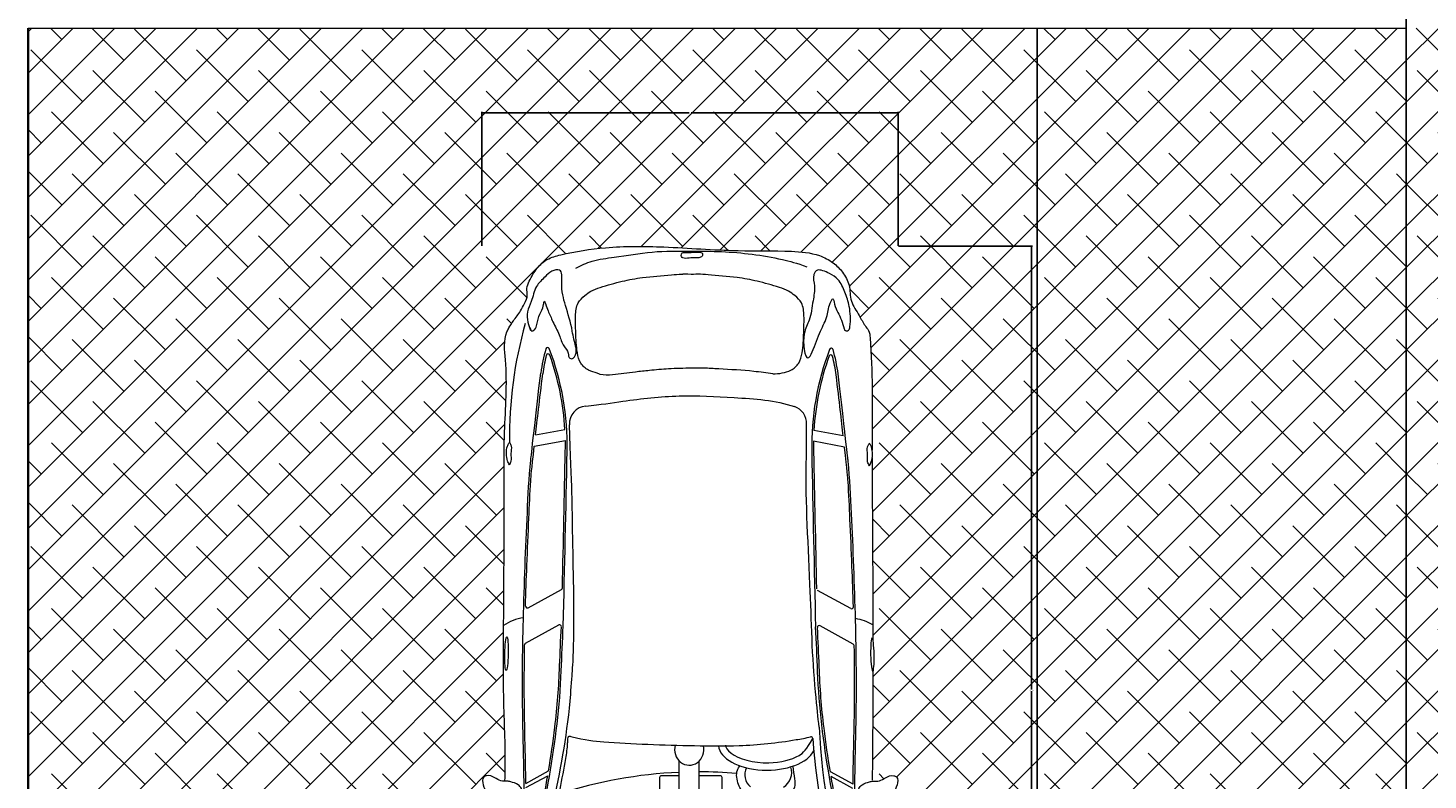
# Model space of a CAD drawing. Units: inches. Extents: x -4843 to -3402, y -164 to 3629.
# Tile 4 of 22: x -4303 to -3999, y 294 to 457. Entities that reach past the tile are written whole.
import ezdxf

# ---------------------------------------------------------------- set-up
doc = ezdxf.new("R2010")
doc.units = ezdxf.units.IN
for name, color, linetype, lineweight in [('A-ANNO-DIMS', 2, 'Continuous', 18), ('C-PRKG-VEHI', 7, 'Continuous', 18), ('C-PVMT', 7, 'Continuous', 18), ('walls', 7, 'Continuous', 35)]:
    doc.layers.add(name, color=color, linetype=linetype, lineweight=lineweight)
doc.layers.add('C-PVMT-PATT', color=9, linetype='Continuous', lineweight=13, true_color=0xc7c8ca)
doc.styles.get("Standard").update_dxf_attribs({"font": 'arial.ttf'})
doc.dimstyles.get("Standard").update_dxf_attribs({"dimtxt": 0.18, "dimasz": 0.18, "dimexe": 0.18, "dimexo": 0.0625, "dimgap": 0.09, "dimtad": 0, "dimtih": 1, "dimtoh": 1, "dimdec": 4, "dimzin": 0, "dimdsep": 46, "dimtxsty": 'Standard', "dimcen": 0.09, "dimadec": 0, "dimazin": 0, "dimtfac": 1, "dimtdec": 4, "dimtofl": 0, "dimtmove": 0, "dimatfit": 3, "dimfxl": 1, "dimtolj": 1, "dimtzin": 0, "dimarcsym": 0})
pattern_1 = [(45, (-7766.296, -1992.247), (-4.490128, 4.490128), []), (135, (-7766.296, -1992.247), (-13.470384, 4.490128), [15.875, -9.525])]

# ---------------------------------------------------------------- blocks, each defined once
blk = doc.blocks.new('A$C3DA776D3')
for p, q in [((1.7076, 1.8326), (1.7664, 1.7249)), ((1.7285, 1.8328), (1.7896, 1.7211)), ((2.4197, 1.8342), (2.5093, 1.6703)), ((2.5943, 1.8214), (2.684, 1.6573)), ((3.3909, 1.7911), (3.4188, 1.6381)), ((3.4459, 1.7849), (3.4724, 1.64)), ((1.6754, 1.0776), (1.84, 1.0776)), ((1.8376, 0.9796), (1.6754, 0.9796)), ((3.3865, 0.2616), (3.4145, 0.4146)), ((2.4153, 0.2185), (2.5049, 0.3824)), ((2.5899, 0.2313), (2.6797, 0.3954)), ((3.4416, 0.2678), (3.468, 0.4127)), ((1.7032, 0.2201), (1.7621, 0.3277)), ((1.7242, 0.2199), (1.7853, 0.3316))]:
    blk.add_line(p, q)
blk.add_lwpolyline([(1.7676, 0.9796), (1.7676, 0.876, -0.414214), (1.7587, 0.8671), (1.6411, 0.8671, -0.414214), (1.6323, 0.876), (1.6323, 1.1626, -0.414214), (1.6411, 1.1715), (1.7587, 1.1715, -0.414214), (1.7676, 1.1626), (1.7676, 1.0776)], format="xyb")
for centre, radius, start, end in [((2.3136, 1.8104), 0.2339, 8.50125, 34.35103), ((3.4366, -0.1255), 2.0392, 74.09296, 90.76485), ((2.4119, 1.83), 0.00887, 28.65835, 89.06838), ((2.6021, 1.8256), 0.00887, 88.34829, 208.65835), ((3.6182, 0.847), 0.9119, 76.0102, 81.87599), ((3.6222, 0.8569), 0.9119, 74.17074, 81.87599), ((3.8365, 1.7232), 0.00887, 289.75061, 76.0102), ((3.8685, 1.7257), 0.00887, 291.10821, 74.17074), ((-0.4678, 0.9763), 2.2529, 2.57809, 17.91043), ((2.5015, 1.6661), 0.00887, 266.38599, 28.65835), ((2.6918, 1.6615), 0.00887, 208.65835, 268.69062), ((3.3971, 2.9469), 1.3179, 268.72162, 291.10821), ((3.3971, 2.9469), 1.309, 273.29531, 289.75061), ((7.8433, 227.0424), 225.4575, 268.64295, 268.862544), ((7.8433, 227.0424), 225.4486, 268.690624, 268.862544), ((3.3971, 2.9469), 1.309, 268.72162, 270.94951), ((3.5001, 1.5294), 0.0887, 5.3633, 92.43356), ((-0.4678, 0.9763), 2.2529, 355.34103, 0.08439), ((1.7703, 0.6782), 0.0753, 62.21447, 141.10294), ((1.782, 0.6059), 0.0837, 210.97226, 288.84464), ((3.5019, 0.5376), 0.0887, 268.70196, 340.8366), ((2.3306, -4.2069), 4.6409, 94.71361, 104.29398), ((1.9485, 0.4271), 0.00887, 274.71361, 10.98745), ((7.8389, -224.9897), 225.4575, 91.137456, 91.35705), ((7.8389, -224.9897), 225.4486, 91.137456, 91.309376), ((3.3928, -0.8942), 1.3179, 68.89179, 91.27838), ((3.3928, -0.8942), 1.309, 89.05049, 91.27838), ((2.1977, -3.2479), 3.6398, 93.02386, 106.34052), ((2.4971, 0.3866), 0.00887, 331.34165, 93.61401), ((3.3928, -0.8942), 1.309, 70.24939, 86.70469), ((3.6138, 1.2057), 0.9119, 278.12401, 283.9898), ((3.6179, 1.1957), 0.9119, 278.12401, 285.82926), ((3.8321, 0.3295), 0.00887, 283.9898, 70.24939), ((3.8642, 0.327), 0.00887, 285.82926, 68.89179), ((2.4075, 0.2227), 0.00887, 270.93162, 331.34165), ((2.3093, 0.2423), 0.2339, 328.98617, 351.49875), ((2.5977, 0.227), 0.00887, 151.34165, 271.65171)]:
    blk.add_arc(centre, radius, start, end)
blk.add_ellipse((2.3672, 1.9283), major_axis=(-0.083, 0.0016), ratio=0.102782)
for centre, major_axis, ratio, start_param, end_param in [((1.8957, 1.0273), (0.0775, 0), 0.932272, 1.29458, 4.948947), ((1.9205, 0.6448), (0, 0.2392), 0.529672, 0.058485, 2.894188)]:
    blk.add_ellipse(centre, major_axis=major_axis, ratio=ratio, start_param=start_param, end_param=end_param)
at = {"extrusion": (0, 0, -1)}
blk.add_ellipse((2.3628, 0.1244), major_axis=(-0.083, -0.0016), ratio=0.102782, dxfattribs=at)
for points, knots in [([(1.633, 1.9421), (1.6372, 1.9559), (1.6485, 1.9865), (1.6785, 2.0254), (1.7174, 2.0443), (1.758, 2.0499), (1.7712, 2.0175), (1.7589, 1.9877), (1.737, 1.958), (1.7418, 1.929), (1.7342, 1.9007), (1.7274, 1.874), (1.7007, 1.849), (1.6682, 1.8516), (1.625, 1.8563), (1.6294, 1.9016), (1.6314, 1.9281), (1.633, 1.9421)], [0.0885943, 0.0885943, 0.0885943, 0.0885943, 0.1373899, 0.1989553, 0.2458559, 0.2904509, 0.3067594, 0.3537167, 0.3919221, 0.4272917, 0.447055, 0.4910496, 0.5184931, 0.5619515, 0.6001709, 0.6402891, 0.6890715, 0.6890715, 0.6890715, 0.6890715]), ([(1.7401, 1.9359), (1.7441, 1.9358), (1.8578, 1.931), (2.1105, 1.9445), (2.4984, 1.9427), (2.8874, 1.9396), (3.2079, 1.9402), (3.5092, 1.9401), (3.7388, 1.9191), (3.9196, 1.945), (3.9792, 1.9134), (4.0141, 1.8916), (4.0511, 1.8608), (4.0944, 1.8389), (4.1316, 1.8213), (4.1705, 1.8314), (4.2164, 1.8107), (4.2677, 1.7817), (4.3166, 1.7281), (4.3472, 1.6107), (4.3777, 1.4199), (4.3756, 1.126), (4.3499, 0.8209), (4.3562, 0.5655), (4.3432, 0.4036), (4.2994, 0.3183), (4.2485, 0.2679), (4.1835, 0.2317), (4.102, 0.2378), (4.0429, 0.19), (3.9911, 0.1682), (3.96, 0.1386), (3.7692, 0.1231), (3.5761, 0.125), (3.3929, 0.1252), (3.3707, 0.1253)], [0.114046, 0.114046, 0.114046, 0.114046, 0.127519, 0.499235, 0.968453, 1.440308, 1.814622, 2.054514, 2.455224, 2.610949, 2.635875, 2.681833, 2.750323, 2.797084, 2.847368, 2.883024, 2.926275, 3.011124, 3.084414, 3.16311, 3.41524, 3.739789, 4.152943, 4.449449, 4.607544, 4.693588, 4.767288, 4.84799, 4.936972, 5.028501, 5.093159, 5.12765, 5.168553, 5.718196, 5.794044, 5.794044, 5.794044, 5.794044]), ([(3.2988, 1.9135), (3.3049, 1.917), (3.3217, 1.9267), (3.3541, 1.9291), (3.3849, 1.9277), (3.4021, 1.9183), (3.4079, 1.9144), (3.4094, 1.9135)], [0, 0, 0, 0, 0.00281353, 0.00784005, 0.01287951, 0.01501274, 0.01570301, 0.01570301, 0.01570301, 0.01570301]), ([(3.2988, 1.9135), (3.3049, 1.91), (3.3217, 1.9002), (3.3541, 1.9083), (3.3849, 1.8992), (3.4021, 1.9086), (3.4079, 1.9125), (3.4094, 1.9135)], [0, 0, 0, 0, 0.00281353, 0.00784005, 0.01287951, 0.01501274, 0.01570301, 0.01570301, 0.01570301, 0.01570301]), ([(1.2647, 1.8108), (1.5866, 1.75), (1.9321, 1.6711), (2.357, 1.6555), (2.4305, 1.6528), (2.5038, 1.6481)], [0.0116221, 0.0116221, 0.0116221, 0.0116221, 0.1543947, 0.1543947, 0.1841997, 0.1841997, 0.1841997, 0.1841997]), ([(1.2695, 1.8548), (1.4293, 1.844), (1.6772, 1.8374), (2.0858, 1.8517), (2.5501, 1.8477), (2.9741, 1.8297), (3.2389, 1.8174), (3.3308, 1.8077), (3.7511, 1.7597)], [0.04998, 0.04998, 0.04998, 0.04998, 0.456658, 0.88886, 1.432548, 2.02833, 2.31987, 2.336539, 2.336539, 2.336539, 2.336539]), ([(1.7285, 1.8328), (1.7747, 1.8334), (1.8206, 1.8343), (1.9706, 1.8377), (2.0741, 1.8401), (2.2558, 1.8407), (2.3339, 1.8401), (2.412, 1.8388)], [0.5222333, 0.5222333, 0.5222333, 0.5222333, 0.6789211, 0.6789211, 1.0296365, 1.0296365, 1.2940564, 1.2940564, 1.2940564, 1.2940564]), ([(2.6023, 1.8345), (2.6692, 1.8326), (2.7361, 1.8303), (2.8806, 1.8247), (2.9582, 1.8213), (3.0971, 1.8151), (3.1585, 1.8125), (3.2439, 1.8067), (3.2678, 1.805), (3.3909, 1.7911)], [1.5086743, 1.5086743, 1.5086743, 1.5086743, 1.734954, 1.734954, 1.9977611, 1.9977611, 2.2072366, 2.2072366, 2.2879509, 2.2879509, 2.2879509, 2.2879509]), ([(3.9734, 1.8117), (3.9663, 1.8096), (3.9533, 1.8057), (3.9675, 1.7837), (3.9974, 1.7757), (4.0449, 1.7671), (4.0687, 1.7469), (4.1118, 1.7427), (4.0814, 1.7311), (4.0537, 1.7221), (3.9987, 1.6973), (3.944, 1.6686), (3.8874, 1.6515), (3.8568, 1.6214), (3.8247, 1.6229), (3.8198, 1.6037), (3.8493, 1.5722), (3.9042, 1.5957), (3.9867, 1.6071), (4.0829, 1.6378), (4.1689, 1.6615), (4.2691, 1.6496), (4.2551, 1.7102), (4.2211, 1.742), (4.177, 1.7897), (4.1098, 1.8), (4.0548, 1.8295), (4.0034, 1.825), (3.9739, 1.8144), (3.9604, 1.8095)], [0, 0, 0, 0, 0.017475, 0.032006, 0.059638, 0.113544, 0.163661, 0.180489, 0.192607, 0.230667, 0.289874, 0.361637, 0.420844, 0.462112, 0.488508, 0.497437, 0.514565, 0.60135, 0.642171, 0.772325, 0.88763, 0.949295, 0.98758, 1.030723, 1.095245, 1.173408, 1.227582, 1.278579, 1.321774, 1.321774, 1.321774, 1.321774]), ([(1.1452, 1.6917), (1.1484, 1.7027), (1.1532, 1.7193), (1.17, 1.7359), (1.1994, 1.7411), (1.2882, 1.7262), (1.4597, 1.7082), (1.664, 1.6726), (1.8239, 1.6391), (1.9094, 1.627), (1.9434, 1.6262), (1.9633, 1.6236), (1.9429, 1.5472), (1.9237, 1.3694), (1.9156, 1.0748), (1.9104, 0.7612), (1.9305, 0.5688), (1.9526, 0.4525), (1.9572, 0.4288)], [0, 0, 0, 0, 0.038062, 0.057765, 0.075887, 0.136118, 0.360736, 0.660851, 0.833831, 0.919425, 0.944413, 0.95681, 0.976133, 1.15453, 1.659168, 1.908025, 2.226872, 2.308645, 2.308645, 2.308645, 2.308645]), ([(1.1477, 1.792), (1.4905, 1.7373), (1.7995, 1.6413), (2.2125, 1.6082), (2.2832, 1.6032), (2.2832, 1.6032)], [0.0003636, 0.0003636, 0.0003636, 0.0003636, 0.134701, 0.134701, 0.1508358, 0.1508358, 0.1508358, 0.1508358]), ([(1.7896, 1.7211), (1.861, 1.7092), (1.9329, 1.6986), (2.1055, 1.6776), (2.2062, 1.67), (2.3721, 1.6638), (2.4366, 1.6613), (2.5009, 1.6572)], [0.08651219, 0.08651219, 0.08651219, 0.08651219, 0.11635961, 0.11635961, 0.15763882, 0.15763882, 0.18372658, 0.18372658, 0.18372658, 0.18372658]), ([(2.2832, 1.6032), (2.3228, 1.5999), (2.5521, 1.5922), (2.8969, 1.602), (3.1915, 1.6051), (3.4964, 1.618)], [0.0364782, 0.0364782, 0.0364782, 0.0364782, 0.0534387, 0.1292772, 0.1736343, 0.1736343, 0.1736343, 0.1736343]), ([(3.7498, 1.4809), (3.754, 1.4954), (3.763, 1.5267), (3.7976, 1.5671), (3.8663, 1.5841), (3.945, 1.586), (4.0264, 1.5897), (4.095, 1.5835), (4.1312, 1.5458), (4.1582, 1.5098), (4.1799, 1.4459), (4.2042, 1.362), (4.2262, 1.2442), (4.2302, 1.1452), (4.2391, 1.0799), (4.2382, 1.0609), (4.238, 1.0593)], [0, 0, 0, 0, 0.051006, 0.109652, 0.169413, 0.283146, 0.376203, 0.448906, 0.503455, 0.546185, 0.600943, 0.729234, 0.842906, 1.005303, 1.062348, 1.067834, 1.067834, 1.067834, 1.067834]), ([(3.5884, 1.5377), (3.5955, 1.4623), (3.6187, 1.3167), (3.6464, 1.0795), (3.6296, 0.7971), (3.6184, 0.6028), (3.5856, 0.5085)], [0.0073838, 0.0073838, 0.0073838, 0.0073838, 0.0294007, 0.067193, 0.1037964, 0.1444788, 0.1444788, 0.1444788, 0.1444788]), ([(4.2687, 1.5864), (4.2814, 1.5601), (4.3101, 1.5003), (4.3237, 1.3708), (4.3542, 1.2092), (4.3516, 1.0314), (4.3515, 0.8166), (4.328, 0.6299), (4.2931, 0.4969), (4.2753, 0.4484)], [0.0003357, 0.0003357, 0.0003357, 0.0003357, 0.0120881, 0.0270745, 0.0525606, 0.0788485, 0.0988506, 0.1397625, 0.1546131, 0.1546131, 0.1546131, 0.1546131]), ([(3.7719, 1.1301), (3.7693, 1.161), (3.7646, 1.2154), (3.755, 1.3075), (3.7437, 1.3871), (3.7385, 1.4523), (3.7479, 1.4761), (3.7498, 1.4809)], [0, 0, 0, 0, 0.0932622, 0.1637418, 0.2771727, 0.3378557, 0.3533593, 0.3533593, 0.3533593, 0.3533593]), ([(3.7464, 0.6151), (3.751, 0.6462), (3.764, 0.7345), (3.7688, 0.849), (3.7776, 0.9708), (3.7739, 1.0537), (3.7724, 1.1114), (3.7719, 1.1301)], [0, 0, 0, 0, 0.0942715, 0.2677429, 0.3431712, 0.4605244, 0.5163856, 0.5163856, 0.5163856, 0.5163856]), ([(3.7464, 0.6151), (3.7487, 0.5841), (3.7523, 0.5353), (3.7976, 0.4824), (3.8663, 0.4655), (3.945, 0.4636), (4.0264, 0.4598), (4.095, 0.4661), (4.1312, 0.5037), (4.1582, 0.5397), (4.1799, 0.6036), (4.2042, 0.6876), (4.2262, 0.8054), (4.2302, 0.9043), (4.2405, 0.9803), (4.2357, 1.0124), (4.2397, 1.0382), (4.238, 1.0593)], [0, 0, 0, 0, 0.102568, 0.161214, 0.220975, 0.334708, 0.427765, 0.500468, 0.555017, 0.597747, 0.652505, 0.780796, 0.894469, 1.056865, 1.11391, 1.156093, 1.160184, 1.160184, 1.160184, 1.160184]), ([(4.3456, 1.0487), (4.3454, 1.055), (4.345, 1.0655), (4.3309, 1.0673), (4.3197, 1.0642), (4.3146, 1.0445), (4.3189, 1.0207), (4.319, 0.9935), (4.3191, 0.9738), (4.3269, 0.9619), (4.3406, 0.9595), (4.3472, 0.9725), (4.3459, 1.0017), (4.3458, 1.0278), (4.3456, 1.0487)], [0, 0, 0, 0, 0.0161503, 0.0269005, 0.0371971, 0.0481428, 0.0821987, 0.1109398, 0.1300767, 0.1391672, 0.1522476, 0.1621518, 0.1776933, 0.2403313, 0.2403313, 0.2403313, 0.2403313]), ([(1.917, 0.8484), (1.9065, 0.8472), (1.8919, 0.8396), (1.8496, 0.7856), (1.8276, 0.7099), (1.8313, 0.5772), (1.8453, 0.5209), (1.8787, 0.4642), (1.8936, 0.4502), (1.9492, 0.4183)], [0.058485, 0.058485, 0.058485, 0.058485, 0.595418, 0.595418, 1.615982, 1.615982, 2.403313, 2.403313, 2.894188, 2.894188, 2.894188, 2.894188]), ([(1.8119, 0.5169), (1.7917, 0.514), (1.7583, 0.5092), (1.7058, 0.5035), (1.6658, 0.5348), (1.6354, 0.5836), (1.6317, 0.6432), (1.632, 0.7046), (1.6686, 0.7545), (1.7219, 0.7885), (1.7812, 0.7994), (1.8082, 0.7822), (1.815, 0.7773)], [0, 0, 0, 0, 0.0697224, 0.1152553, 0.1718464, 0.228887, 0.3065165, 0.3695628, 0.4317857, 0.5044965, 0.584817, 0.6125638, 0.6125638, 0.6125638, 0.6125638]), ([(2.0057, 0.3869), (2.0557, 0.3932), (2.0992, 0.3965), (2.3523, 0.4219), (2.5289, 0.4244), (2.9365, 0.4421), (3.1622, 0.4555), (3.3596, 0.4486), (3.3948, 0.4513), (3.4999, 0.4489)], [0.1070055, 0.1070055, 0.1070055, 0.1070055, 0.1399042, 0.1399042, 0.2098563, 0.2098563, 0.2979905, 0.2979905, 0.3093168, 0.3093168, 0.3093168, 0.3093168]), ([(3.964, 0.2612), (3.9617, 0.2588), (3.9566, 0.2535), (3.9614, 0.2383), (3.9909, 0.2329), (4.0293, 0.2321), (4.0884, 0.2378), (4.1495, 0.2578), (4.2101, 0.2858), (4.2415, 0.3309), (4.2547, 0.3649), (4.2635, 0.3979), (4.2268, 0.4216), (4.1745, 0.4036), (4.1001, 0.4199), (4.0156, 0.4277), (3.9418, 0.4747), (3.7655, 0.4508), (3.9022, 0.4031), (3.965, 0.3781), (4.0329, 0.3413), (4.0824, 0.3422), (4.1256, 0.3165), (4.078, 0.3105), (4.0424, 0.2885), (3.9952, 0.269), (3.9647, 0.2624), (3.9625, 0.2619)], [0, 0, 0, 0, 0.009236, 0.020978, 0.038973, 0.091268, 0.140769, 0.214303, 0.284815, 0.335662, 0.372324, 0.398893, 0.425844, 0.481921, 0.555683, 0.652944, 0.723836, 0.844841, 0.937264, 0.99125, 1.075051, 1.147232, 1.161311, 1.187896, 1.23204, 1.31879, 1.325771, 1.325771, 1.325771, 1.325771]), ([(1.2603, 0.2419), (1.5822, 0.3027), (1.9277, 0.3816), (2.3526, 0.3972), (2.4261, 0.3999), (2.4995, 0.4046)], [0.0116221, 0.0116221, 0.0116221, 0.0116221, 0.1543947, 0.1543947, 0.1841997, 0.1841997, 0.1841997, 0.1841997]), ([(1.7853, 0.3316), (1.8566, 0.3435), (1.9286, 0.3541), (2.1011, 0.3751), (2.2018, 0.3827), (2.3678, 0.3889), (2.4322, 0.3914), (2.4966, 0.3955)], [0.08651219, 0.08651219, 0.08651219, 0.08651219, 0.11635961, 0.11635961, 0.15763882, 0.15763882, 0.18372658, 0.18372658, 0.18372658, 0.18372658]), ([(1.2651, 0.1979), (1.425, 0.2087), (1.6729, 0.2152), (2.0815, 0.2009), (2.5458, 0.205), (2.9697, 0.2229), (3.2345, 0.2353), (3.3264, 0.245), (3.7467, 0.293)], [0.04998, 0.04998, 0.04998, 0.04998, 0.456658, 0.88886, 1.432548, 2.02833, 2.31987, 2.336539, 2.336539, 2.336539, 2.336539]), ([(1.7242, 0.2199), (1.7704, 0.2193), (1.8163, 0.2184), (1.9663, 0.215), (2.0698, 0.2126), (2.2514, 0.212), (2.3295, 0.2126), (2.4077, 0.2138)], [0.5222333, 0.5222333, 0.5222333, 0.5222333, 0.6789211, 0.6789211, 1.0296365, 1.0296365, 1.2940564, 1.2940564, 1.2940564, 1.2940564]), ([(2.598, 0.2182), (2.6649, 0.2201), (2.7318, 0.2224), (2.8763, 0.228), (2.9538, 0.2314), (3.0928, 0.2376), (3.1541, 0.2402), (3.2395, 0.246), (3.2635, 0.2477), (3.3865, 0.2616)], [1.5086743, 1.5086743, 1.5086743, 1.5086743, 1.734954, 1.734954, 1.9977611, 1.9977611, 2.2072366, 2.2072366, 2.2879509, 2.2879509, 2.2879509, 2.2879509]), ([(1.6314, 0.1164), (1.6344, 0.0983), (1.6457, 0.0631), (1.6785, 0.0206), (1.7174, 0.0016), (1.758, -0.0039), (1.7712, 0.0285), (1.7589, 0.0583), (1.737, 0.0879), (1.7418, 0.117), (1.7342, 0.1453), (1.7274, 0.1719), (1.7007, 0.197), (1.6682, 0.1944), (1.625, 0.1897), (1.6289, 0.1495), (1.6307, 0.1265), (1.6314, 0.1164)], [0.0739443, 0.0739443, 0.0739443, 0.0739443, 0.1373899, 0.1989553, 0.2458559, 0.2904509, 0.3067594, 0.3537167, 0.3919221, 0.4272917, 0.447055, 0.4910496, 0.5184931, 0.5619515, 0.6001709, 0.6402891, 0.6746905, 0.6746905, 0.6746905, 0.6746905]), ([(3.2944, 0.1392), (3.3005, 0.1427), (3.3174, 0.1525), (3.3498, 0.1444), (3.3806, 0.1535), (3.3978, 0.1441), (3.4036, 0.1402), (3.405, 0.1392)], [0, 0, 0, 0, 0.00281353, 0.00784005, 0.01287951, 0.01501274, 0.01570301, 0.01570301, 0.01570301, 0.01570301]), ([(3.2944, 0.1392), (3.3005, 0.1357), (3.3174, 0.126), (3.3498, 0.1236), (3.3806, 0.125), (3.3978, 0.1344), (3.4036, 0.1383), (3.405, 0.1392)], [0, 0, 0, 0, 0.00281353, 0.00784005, 0.01287951, 0.01501274, 0.01570301, 0.01570301, 0.01570301, 0.01570301])]:
    blk.add_open_spline(points, degree=3, knots=knots)
for points in [[(1.4148, 1.7908), (1.5298, 1.7683), (1.6473, 1.7451), (1.7664, 1.7249)], [(3.4459, 1.7849), (3.5176, 1.7767), (3.6145, 1.7654), (3.747, 1.7497)], [(1.4105, 0.2619), (1.5255, 0.2844), (1.6429, 0.3076), (1.7621, 0.3277)], [(3.4416, 0.2678), (3.5133, 0.276), (3.6101, 0.2873), (3.7427, 0.303)], [(2.2804, 0.1218), (2.1011, 0.1222), (1.9224, 0.1236), (1.7436, 0.125)], [(3.333, 0.1253), (3.0361, 0.1252), (2.7351, 0.1219), (2.4353, 0.1216)]]:
    blk.add_open_spline(points, degree=3)
blk = doc.blocks.new('*D58')
at = {"layer": 'A-ANNO-DIMS', "color": 0, "lineweight": -2, "transparency": 16777216}
for p, q in [((-4113.85, 410.04), (-4084.81, 410.04)), ((-4084.99, 409.86), (-4084.99, 313.81)), ((-4084.99, 217.38), (-4084.99, 313.44)), ((-4113.85, 217.2), (-4084.81, 217.2))]:
    blk.add_line(p, q, dxfattribs=at)
at = {"layer": 'A-ANNO-DIMS', "color": 0, "transparency": 16777216}
for points in [[(-4085.02, 409.86), (-4084.96, 409.86), (-4084.99, 410.04)], [(-4085.02, 217.38), (-4084.96, 217.38), (-4084.99, 217.2)]]:
    blk.add_solid(points, dxfattribs=at)
at = {"layer": 'Defpoints', "color": 0, "transparency": 16777216}
for p in [(-4113.92, 410.04), (-4084.99, 410.04), (-4113.92, 217.2)]:
    blk.add_point(p, dxfattribs=at)
at = {"layer": 'A-ANNO-DIMS', "color": 0, "transparency": 16777216, "insert": (-4084.99, 313.62), "char_height": 0.18, "attachment_point": 5}
blk.add_mtext('\\A1;CAR 193', dxfattribs=at)
blk = doc.blocks.new('*D59')
at = {"layer": 'A-ANNO-DIMS', "color": 0, "lineweight": -2, "transparency": 16777216}
for p, q in [((-4204.26, 410.11), (-4204.26, 439.15)), ((-4204.08, 438.97), (-4159.3, 438.97)), ((-4114.1, 438.97), (-4158.87, 438.97)), ((-4113.92, 410.11), (-4113.92, 439.15))]:
    blk.add_line(p, q, dxfattribs=at)
at = {"layer": 'A-ANNO-DIMS', "color": 0, "transparency": 16777216}
for points in [[(-4204.08, 439), (-4204.08, 438.94), (-4204.26, 438.97)], [(-4114.1, 439), (-4114.1, 438.94), (-4113.92, 438.97)]]:
    blk.add_solid(points, dxfattribs=at)
at = {"layer": 'Defpoints', "color": 0, "transparency": 16777216}
for p in [(-4204.26, 438.97), (-4204.26, 410.04), (-4113.92, 410.04)]:
    blk.add_point(p, dxfattribs=at)
at = {"layer": 'A-ANNO-DIMS', "color": 0, "transparency": 16777216, "insert": (-4159.09, 438.97), "char_height": 0.18, "attachment_point": 5}
blk.add_mtext('\\A1;90', dxfattribs=at)
blk = doc.blocks.new('*D63')
at = {"layer": 'A-ANNO-DIMS', "color": 0, "lineweight": -2, "transparency": 16777216}
for p, q in [((-4083.78, 457.29), (-4083.78, 10.92)), ((-4302.78, 275.29), (-4302.78, 10.92)), ((-4302.6, 11.1), (-4193.57, 11.1)), ((-4083.96, 11.1), (-4192.99, 11.1))]:
    blk.add_line(p, q, dxfattribs=at)
at = {"layer": 'A-ANNO-DIMS', "color": 0, "transparency": 16777216}
for points in [[(-4302.6, 11.13), (-4302.6, 11.07), (-4302.78, 11.1)], [(-4083.96, 11.13), (-4083.96, 11.07), (-4083.78, 11.1)]]:
    blk.add_solid(points, dxfattribs=at)
at = {"layer": 'Defpoints', "color": 0, "transparency": 16777216}
for p in [(-4083.78, 457.35), (-4302.78, 275.35), (-4083.78, 11.1)]:
    blk.add_point(p, dxfattribs=at)
at = {"layer": 'A-ANNO-DIMS', "color": 0, "transparency": 16777216, "insert": (-4193.28, 11.1), "char_height": 0.18, "attachment_point": 5}
blk.add_mtext('\\A1;219', dxfattribs=at)
blk = doc.blocks.new('*D66')
at = {"layer": 'A-ANNO-DIMS', "color": 0, "lineweight": -2, "transparency": 16777216}
for p, q in [((-4083.78, 457.29), (-4083.78, 10.92)), ((-3941.78, 86.29), (-3941.78, 10.92)), ((-4083.6, 11.1), (-4013.06, 11.1)), ((-3941.96, 11.1), (-4012.5, 11.1))]:
    blk.add_line(p, q, dxfattribs=at)
at = {"layer": 'A-ANNO-DIMS', "color": 0, "transparency": 16777216}
for points in [[(-4083.6, 11.13), (-4083.6, 11.07), (-4083.78, 11.1)], [(-3941.96, 11.13), (-3941.96, 11.07), (-3941.78, 11.1)]]:
    blk.add_solid(points, dxfattribs=at)
at = {"layer": 'Defpoints', "color": 0, "transparency": 16777216}
for p in [(-4083.78, 457.35), (-3941.78, 86.35), (-3941.78, 11.1)]:
    blk.add_point(p, dxfattribs=at)
at = {"layer": 'A-ANNO-DIMS', "color": 0, "transparency": 16777216, "insert": (-4012.78, 11.1), "char_height": 0.18, "attachment_point": 5}
blk.add_mtext('\\A1;142', dxfattribs=at)
blk = doc.blocks.new('*D81')
at = {"layer": 'A-ANNO-DIMS', "color": 0, "lineweight": -2, "transparency": 16777216}
for p, q in [((-4332.78, 86.42), (-4332.78, 1392.95)), ((-4332.6, 1392.77), (-4168.61, 1392.77)), ((-4003.86, 1392.77), (-4167.86, 1392.77)), ((-4003.68, 86.42), (-4003.68, 1392.95))]:
    blk.add_line(p, q, dxfattribs=at)
at = {"layer": 'A-ANNO-DIMS', "color": 0, "transparency": 16777216}
for points in [[(-4332.6, 1392.8), (-4332.6, 1392.74), (-4332.78, 1392.77)], [(-4003.86, 1392.8), (-4003.86, 1392.74), (-4003.68, 1392.77)]]:
    blk.add_solid(points, dxfattribs=at)
at = {"layer": 'Defpoints', "color": 0, "transparency": 16777216}
for p in [(-4003.68, 1392.77), (-4332.78, 86.35), (-4003.68, 86.35)]:
    blk.add_point(p, dxfattribs=at)
at = {"layer": 'A-ANNO-DIMS', "color": 0, "transparency": 16777216, "insert": (-4168.23, 1392.77), "char_height": 0.18, "attachment_point": 5}
blk.add_mtext('\\A1;329.1', dxfattribs=at)

msp = doc.modelspace()

# ---------------------------------------------------------------- hatches: boundary and pattern name
at = {"layer": 'C-PVMT-PATT'}
h = msp.add_hatch(dxfattribs=at)
h.set_pattern_fill('ANSI38', color=256, scale=2)
h.set_pattern_definition(pattern_1)
h.paths.add_polyline_path([(-4583.98, 275.35), (-4595.78, 275.35), (-4595.78, 324.35), (-4595.78, 373.35), (-4595.78, 466.35), (-4696.78, 466.35), (-4696.78, 95.35), (-4583.98, 95.35), (-4583.98, 226.6)])
h.paths.add_polyline_path([(-4302.78, 226.6), (-4583.98, 226.6), (-4583.98, 95.35), (-4332.78, 95.35), (-4332.78, 86.35), (-4003.68, 86.35), (-4003.68, 95.35), (-3978.78, 95.35), (-3978.78, 457.35), (-4003.68, 457.35), (-4003.68, 139.54), (-4302.78, 139.54)])
h = msp.add_hatch(dxfattribs=at)
h.set_pattern_fill('ANSI38', color=256, scale=2)
h.set_pattern_definition(pattern_1)
h.paths.add_polyline_path([(-4302.78, 139.54), (-4003.68, 139.54), (-4003.68, 457.35), (-4302.78, 457.35)])
edge = h.paths.add_edge_path(flags=16)
edge.add_spline(control_points=[(-4177.52, 219.09), (-4179, 219.51), (-4181.86, 220.31), (-4185.82, 220.95), (-4189.05, 222.54), (-4192.16, 223.72), (-4194.07, 225.9), (-4195.4, 228.28), (-4195.62, 231.06), (-4195.51, 234.52), (-4196.21, 237.87), (-4197.78, 240.97), (-4199.51, 244.96), (-4199.58, 253.67), (-4199.59, 264.61), (-4199.42, 277.52), (-4199.5, 285.22), (-4199.55, 289.24)], knot_values=[0, 0, 0, 0, 0.118823, 0.228347, 0.304709, 0.395218, 0.479661, 0.520666, 0.602694, 0.688012, 0.788383, 0.860898, 0.954729, 1.11959, 1.518327, 1.801929, 2.110556, 2.110556, 2.110556, 2.110556], degree=3, periodic=0)
edge.add_spline(control_points=[(-4199.55, 289.24), (-4200.15, 289.43), (-4201.5, 289.92), (-4203.22, 291.24), (-4204.05, 292.95), (-4204.29, 294.74), (-4202.87, 295.32), (-4201.55, 294.78), (-4200.39, 293.92), (-4199.58, 293.95), (-4199.28, 293.95)], knot_values=[0.088594, 0.088594, 0.088594, 0.088594, 0.13739, 0.198955, 0.245856, 0.290451, 0.306759, 0.353717, 0.391922, 0.414753, 0.414753, 0.414753, 0.414753], degree=3, periodic=0)
edge.add_spline(control_points=[(-4199.28, 293.95), (-4199.27, 294.13), (-4199.06, 299.13), (-4199.65, 310.26), (-4199.6, 321.33), (-4199.56, 327.57), (-4199.56, 327.7)], knot_values=[0.114046, 0.114046, 0.114046, 0.114046, 0.127519, 0.499235, 0.968453, 0.97871, 0.97871, 0.97871, 0.97871], degree=3, periodic=0)
edge.add_spline(control_points=[(-4199.56, 327.7), (-4199.52, 333.71), (-4199.44, 344.59), (-4199.46, 358.57), (-4199.46, 371.83), (-4198.54, 381.94), (-4199.67, 389.9), (-4198.28, 392.53), (-4197.33, 394.06), (-4195.97, 395.69), (-4195, 397.6), (-4194.23, 399.23), (-4194.68, 400.94), (-4193.76, 402.97), (-4192.49, 405.22), (-4190.13, 407.38), (-4184.96, 408.73), (-4176.56, 410.07), (-4163.62, 409.97), (-4150.19, 408.84), (-4138.94, 409.12), (-4131.82, 408.55), (-4128.06, 406.62), (-4125.85, 404.38), (-4124.25, 401.52), (-4124.52, 397.93), (-4122.42, 395.33), (-4121.46, 393.05), (-4120.15, 391.68), (-4119.47, 383.28), (-4119.55, 374.78), (-4119.57, 366.71), (-4119.57, 365.74)], knot_values=[0.97871, 0.97871, 0.97871, 0.97871, 1.440308, 1.814622, 2.054514, 2.455224, 2.610949, 2.635875, 2.681833, 2.750323, 2.797084, 2.847368, 2.883024, 2.926275, 3.011124, 3.084414, 3.16311, 3.41524, 3.739789, 4.152943, 4.449449, 4.607544, 4.693588, 4.767288, 4.84799, 4.936972, 5.028501, 5.093159, 5.12765, 5.168553, 5.718196, 5.794044, 5.794044, 5.794044, 5.794044], degree=3, periodic=0)
edge.add_spline(control_points=[(-4120.18, 367.25), (-4120.14, 367.18), (-4119.97, 366.93), (-4119.55, 366.17), (-4119.49, 364.82), (-4119.6, 363.39), (-4120.03, 362.65), (-4120.18, 362.38)], knot_values=[0, 0, 0, 0, 0.00069, 0.002823, 0.007863, 0.012889, 0.015703, 0.015703, 0.015703, 0.015703], degree=3, periodic=0)
edge.add_spline(control_points=[(-4119.57, 364.08), (-4119.56, 351.01), (-4119.42, 337.76), (-4119.41, 324.56)], knot_values=[5.836848, 5.836848, 5.836848, 5.836848, 6.848265, 6.848265, 6.848265, 6.848265], degree=3, periodic=0)
edge.add_ellipse((-4119.53, 321.37), major_axis=(-0.07, 3.66), ratio=0.102782, start_angle=-179.3184, end_angle=-3.3021, ccw=False)
edge.add_spline(control_points=[(-4119.41, 317.74), (-4119.43, 309.85), (-4119.49, 301.98), (-4119.55, 294.11)], knot_values=[7.022686, 7.022686, 7.022686, 7.022686, 7.62832, 7.62832, 7.62832, 7.62832], degree=3, periodic=0)
edge.add_spline(control_points=[(-4119.55, 294.11), (-4119.55, 294.04), (-4119.54, 293.98), (-4119.53, 293.92)], knot_values=[3.166598, 3.166598, 3.166598, 3.166598, 3.17144, 3.17144, 3.17144, 3.17144], degree=3, periodic=0)
edge.add_spline(control_points=[(-4119.53, 293.92), (-4119.49, 293.93), (-4118.98, 293.99), (-4117.92, 293.82), (-4116.62, 294.78), (-4115.3, 295.32), (-4113.88, 294.74), (-4114.12, 292.95), (-4114.96, 291.24), (-4116.83, 289.8), (-4118.38, 289.3), (-4119.18, 289.17)], knot_values=[0.073944, 0.073944, 0.073944, 0.073944, 0.077675, 0.113045, 0.15125, 0.198208, 0.214516, 0.259111, 0.306012, 0.367577, 0.431023, 0.431023, 0.431023, 0.431023], degree=3, periodic=0)
edge.add_spline(control_points=[(-4119.18, 289.17), (-4119.16, 288.25), (-4119.23, 285.31), (-4120.26, 281.21), (-4116.4, 269.66), (-4119.27, 257.62), (-4120.12, 246.29), (-4120, 242.31), (-4122.07, 238.8), (-4123.28, 234.04), (-4123.32, 229.29), (-4124.68, 225.36), (-4128.1, 222.41), (-4132.86, 220.91), (-4139.06, 219.63), (-4143.16, 218.66), (-4145.64, 218.22)], knot_values=[0.819302, 0.819302, 0.819302, 0.819302, 0.890194, 1.044711, 1.132212, 1.809474, 1.943489, 2.01252, 2.108859, 2.247504, 2.386276, 2.473581, 2.556705, 2.722147, 2.850835, 3.044752, 3.044752, 3.044752, 3.044752], degree=3, periodic=0)
edge.add_spline(control_points=[(-4145.64, 218.22), (-4146.33, 218.09), (-4151.86, 217.2), (-4162, 217.3), (-4171.27, 218.35), (-4175.68, 218.87)], knot_values=[0.047426, 0.047426, 0.047426, 0.047426, 0.101273, 0.477921, 0.819302, 0.819302, 0.819302, 0.819302], degree=3, periodic=0)
edge.add_spline(control_points=[(-4175.68, 218.87), (-4176.29, 218.95), (-4176.91, 219.02), (-4177.52, 219.09)], knot_values=[0, 0, 0, 0, 0.047426, 0.047426, 0.047426, 0.047426], degree=3, periodic=0)
edge = h.paths.add_edge_path(flags=0)
edge.add_spline(control_points=[(-4193.77, 273.03), (-4191.09, 287.2), (-4187.62, 302.4), (-4186.93, 321.11), (-4186.81, 324.35), (-4186.61, 327.58)], knot_values=[0.011622, 0.011622, 0.011622, 0.011622, 0.154395, 0.154395, 0.1842, 0.1842, 0.1842, 0.1842], degree=3, periodic=0)
edge.add_arc((-14109, 562.63), 9925.18, 358.64295, 358.862544)
edge.add_arc((-4243.78, 366.9), 58.02, 358.7216, 381.1082)
edge.add_arc((-4190.02, 387.65), 0.39, 21.1082, 164.1707)
edge.add_arc((-4151.78, 376.81), 40.14, 164.1707, 171.876)
edge.add_spline(control_points=[(-4191.52, 382.48), (-4193.63, 363.98), (-4194.06, 359.93), (-4194.6, 348.28), (-4195.39, 329.61), (-4195.57, 309.17), (-4194.94, 291.19), (-4195.23, 280.27), (-4195.7, 273.24)], knot_values=[0.04998, 0.04998, 0.04998, 0.04998, 0.066649, 0.35819, 0.953971, 1.497659, 1.929861, 2.336539, 2.336539, 2.336539, 2.336539], degree=3, periodic=0)
edge.add_arc((-4194.73, 273.21), 0.976, 178.3008, 349.1958)
edge = h.paths.add_edge_path(flags=0)
edge.add_spline(control_points=[(-4195.31, 273.22), (-4195.21, 274.79), (-4195.12, 276.28), (-4195.04, 277.7)], knot_values=[0.050139, 0.050139, 0.050139, 0.050139, 0.140986, 0.140986, 0.140986, 0.140986], degree=3, periodic=0)
edge.add_line((-4195.04, 277.7), (-4193.1, 278.54))
edge.add_spline(control_points=[(-4193.1, 278.54), (-4193.46, 276.71), (-4193.81, 274.9), (-4194.15, 273.1)], knot_values=[0.011622, 0.011622, 0.011622, 0.011622, 0.029731, 0.029731, 0.029731, 0.029731], degree=3, periodic=0)
edge.add_arc((-4194.73, 273.21), 0.586, 178.9277, 349.1656, ccw=False)
edge = h.paths.add_edge_path(flags=0)
edge.add_spline(control_points=[(-4192.94, 267.88), (-4190.53, 282.97), (-4186.3, 296.57), (-4184.85, 314.75), (-4184.63, 317.86), (-4184.63, 317.86)], knot_values=[0.000364, 0.000364, 0.000364, 0.000364, 0.134701, 0.134701, 0.150836, 0.150836, 0.150836, 0.150836], degree=3, periodic=0)
edge.add_spline(control_points=[(-4184.63, 317.86), (-4184.48, 319.61), (-4184.14, 329.7), (-4184.58, 344.88), (-4184.71, 357.85), (-4185.28, 371.27)], knot_values=[0.036478, 0.036478, 0.036478, 0.036478, 0.053439, 0.129277, 0.173634, 0.173634, 0.173634, 0.173634], degree=3, periodic=0)
edge.add_arc((-4181.38, 371.43), 3.9, 95.3633, 182.3534, ccw=False)
edge.add_spline(control_points=[(-4181.75, 375.32), (-4178.43, 375.63), (-4172.02, 376.65), (-4161.57, 377.87), (-4149.14, 377.13), (-4140.59, 376.64), (-4136.44, 375.2)], knot_values=[0.007384, 0.007384, 0.007384, 0.007384, 0.029401, 0.067193, 0.103796, 0.144479, 0.144479, 0.144479, 0.144479], degree=3, periodic=0)
edge.add_arc((-4137.72, 371.51), 3.9, -1.298, 70.8366, ccw=False)
edge.add_spline(control_points=[(-4133.81, 371.42), (-4133.92, 366.8), (-4133.8, 365.25), (-4134.1, 356.56), (-4133.51, 346.62), (-4132.74, 328.68), (-4132.62, 320.9), (-4131.51, 309.76), (-4131.36, 307.85), (-4131.08, 305.65)], knot_values=[0.107006, 0.107006, 0.107006, 0.107006, 0.118332, 0.118332, 0.206466, 0.206466, 0.276418, 0.276418, 0.309317, 0.309317, 0.309317, 0.309317], degree=3, periodic=0)
edge.add_arc((-3971.07, 314.1), 160.23, 183.0239, 196.3405)
edge.add_arc((-4128.58, 267.92), 3.9, -60.024, 16.3405, ccw=False)
edge.add_arc((-4159.42, 321.39), 65.63, 241.2771, 299.976, ccw=False)
edge.add_arc((-4189.08, 267.26), 3.9, 170.9279, 241.2771, ccw=False)
edge = h.paths.add_edge_path(flags=0)
edge.add_spline(control_points=[(-4194.99, 278.72), (-4194.87, 281.24), (-4194.79, 283.56), (-4194.71, 288.07), (-4194.71, 290.31), (-4194.73, 292.52)], knot_values=[0.163087, 0.163087, 0.163087, 0.163087, 0.328206, 0.328206, 0.498586, 0.498586, 0.498586, 0.498586], degree=3, periodic=0)
edge.add_line((-4194.73, 292.52), (-4189.99, 295.11))
edge.add_spline(control_points=[(-4189.99, 295.11), (-4190.88, 289.87), (-4191.9, 284.7), (-4192.89, 279.64)], knot_values=[0.033336, 0.033336, 0.033336, 0.033336, 0.083278, 0.083278, 0.083278, 0.083278], degree=3, periodic=0)
edge.add_line((-4192.89, 279.64), (-4194.99, 278.72))
edge = h.paths.add_edge_path(flags=0)
edge.add_spline(control_points=[(-4178.7, 221.84), (-4179.39, 222.03), (-4180.88, 222.44), (-4183.38, 222.93), (-4185.9, 223.59), (-4189.06, 224.07), (-4191.51, 226.12), (-4193.19, 228.61), (-4194.59, 231.18), (-4194.2, 234.35), (-4194.53, 237.78), (-4194.39, 240.52), (-4195.15, 242.77), (-4194.42, 243.88), (-4193.69, 245.31), (-4192.7, 244.3), (-4192.76, 242.61), (-4192.13, 240.02), (-4191.54, 236.65), (-4189.84, 233.5), (-4187.61, 230.62), (-4184.55, 228.88), (-4182.1, 227.6), (-4180.18, 227.57), (-4179.35, 226.59), (-4178.67, 225.18), (-4178.52, 223.73), (-4177.56, 222.16), (-4178.35, 221.94), (-4178.7, 221.84)], knot_values=[0, 0, 0, 0, 0.048183, 0.105687, 0.173148, 0.226645, 0.320656, 0.377708, 0.433539, 0.514499, 0.587235, 0.668333, 0.704408, 0.73448, 0.764541, 0.77911, 0.812729, 0.87811, 0.959931, 1.044551, 1.119493, 1.20463, 1.28096, 1.307559, 1.326943, 1.363733, 1.411478, 1.437083, 1.45761, 1.45761, 1.45761, 1.45761], degree=3, periodic=0)
edge = h.paths.add_edge_path(flags=0)
edge.add_spline(control_points=[(-4188.52, 267.77), (-4189.01, 267.9), (-4189.74, 268.12), (-4190.47, 268.86), (-4190.7, 270.15), (-4190.08, 273.88), (-4189.7, 277.37), (-4189.34, 280.09)], knot_values=[0, 0, 0, 0, 0.038062, 0.057765, 0.075887, 0.136118, 0.346676, 0.346676, 0.346676, 0.346676], degree=3, periodic=0)
edge.add_spline(control_points=[(-4189.34, 280.09), (-4189.32, 280.27), (-4188.86, 283.67), (-4188.3, 287.07), (-4187.7, 290.25)], knot_values=[0.346676, 0.346676, 0.346676, 0.346676, 0.360736, 0.61029, 0.61029, 0.61029, 0.61029], degree=3, periodic=0)
edge.add_spline(control_points=[(-4187.7, 290.25), (-4187.64, 290.55), (-4187.59, 290.84), (-4187.53, 291.13)], knot_values=[0.61029, 0.61029, 0.61029, 0.61029, 0.63318, 0.63318, 0.63318, 0.63318], degree=3, periodic=0)
edge.add_spline(control_points=[(-4187.53, 291.13), (-4187.46, 291.48), (-4186.97, 294.04), (-4186.21, 297.64), (-4185.68, 301.41), (-4185.64, 302.9), (-4185.53, 303.78), (-4182.16, 302.88), (-4174.34, 302.04), (-4164.13, 301.75), (-4156.84, 301.61), (-4156.19, 301.6)], knot_values=[0.63318, 0.63318, 0.63318, 0.63318, 0.660851, 0.833831, 0.919425, 0.944413, 0.95681, 0.976133, 1.15453, 1.659168, 1.709179, 1.709179, 1.709179, 1.709179], degree=3, periodic=0)
edge.add_spline(control_points=[(-4156.19, 301.6), (-4155.1, 301.58), (-4154.03, 301.57), (-4152.95, 301.57)], knot_values=[1.709179, 1.709179, 1.709179, 1.709179, 1.79199, 1.79199, 1.79199, 1.79199], degree=3, periodic=0)
edge.add_spline(control_points=[(-4152.95, 301.57), (-4152.42, 301.57), (-4151.9, 301.57), (-4151.37, 301.57)], knot_values=[1.79199, 1.79199, 1.79199, 1.79199, 1.832683, 1.832683, 1.832683, 1.832683], degree=3, periodic=0)
edge.add_spline(control_points=[(-4151.37, 301.57), (-4150.4, 301.58), (-4145.3, 301.69), (-4139.09, 302.34), (-4133.97, 303.31), (-4132.93, 303.51)], knot_values=[1.832683, 1.832683, 1.832683, 1.832683, 1.908025, 2.226872, 2.308645, 2.308645, 2.308645, 2.308645], degree=3, periodic=0)
edge.add_arc((-4132.85, 303.13), 0.39, 4.7136, 100.9875, ccw=False)
edge.add_arc((-3928.85, 319.95), 204.3, 184.7136, 194.294)
edge.add_arc((-4127.21, 269.41), 0.39, -17.7257, 14.294, ccw=False)
edge.add_spline(control_points=[(-4126.84, 269.29), (-4126.85, 269.25), (-4126.95, 268.96), (-4127.33, 268.39), (-4128.31, 268.05), (-4128.95, 267.71), (-4129.3, 267.52)], knot_values=[0, 0, 0, 0, 0.003035, 0.023811, 0.049681, 0.080112, 0.080112, 0.080112, 0.080112], degree=3, periodic=0)
edge.add_spline(control_points=[(-4129.3, 267.52), (-4133.15, 266.24), (-4140.45, 263.81), (-4151.73, 262.21), (-4163.24, 261.98), (-4173.69, 262.83), (-4182.22, 265.35), (-4186.54, 267.01), (-4188.52, 267.77)], knot_values=[0, 0, 0, 0, 0.276247, 0.522812, 0.772814, 1.060937, 1.232089, 1.37667, 1.37667, 1.37667, 1.37667], degree=3, periodic=0)
edge = h.paths.add_edge_path(flags=0)
edge.add_spline(control_points=[(-4194.74, 293.44), (-4194.76, 295.48), (-4194.8, 297.5), (-4194.95, 304.1), (-4195.06, 308.66), (-4195.08, 316.65), (-4195.06, 320.09), (-4195, 323.53)], knot_values=[0.522233, 0.522233, 0.522233, 0.522233, 0.678921, 0.678921, 1.029636, 1.029636, 1.294056, 1.294056, 1.294056, 1.294056], degree=3, periodic=0)
edge.add_arc((-4194.61, 323.53), 0.39, 118.6584, 180.1243, ccw=False)
edge.add_line((-4194.8, 323.87), (-4187.58, 327.81))
edge.add_arc((-4187.4, 327.47), 0.39, -1.7955, 118.6584, ccw=False)
edge.add_spline(control_points=[(-4187.01, 327.45), (-4187.19, 324.61), (-4187.3, 321.78), (-4187.57, 314.47), (-4187.91, 310.04), (-4188.83, 302.44), (-4189.3, 299.28), (-4189.82, 296.13)], knot_values=[0.086512, 0.086512, 0.086512, 0.086512, 0.1126, 0.1126, 0.153879, 0.153879, 0.183727, 0.183727, 0.183727, 0.183727], degree=3, periodic=0)
edge.add_line((-4189.82, 296.13), (-4194.74, 293.44))
h.paths.add_polyline_path([(-4186.78, 287.12, -0.033695), (-4130.99, 288.38, -0.199929), (-4148.63, 273.2), (-4148.83, 271.67, -0.261093), (-4149.06, 271.36, -0.216615), (-4169.29, 271.5, -0.246093), (-4169.52, 271.79), (-4169.81, 273.49, -0.273701)], flags=0)
edge = h.paths.add_edge_path(flags=0)
edge.add_arc((-4140.72, 295.8), 3.69, -59.0277, 20.0091, ccw=False)
edge.add_arc((-4142.47, 285.34), 8.16, 63.4848, 115.5347)
edge.add_arc((-4143.91, 295.28), 3.32, 152.2145, 231.1029, ccw=False)
edge.add_ellipse((-4142.44, 301.89), major_axis=(10.53, 0), ratio=0.529672, start_angle=218.5261, end_angle=229.0127, ccw=False)
edge.add_spline(control_points=[(-4148.27, 297.25), (-4148.49, 296.95), (-4148.81, 296.44), (-4148.95, 295.85), (-4148.97, 295.61)], knot_values=[0.565799, 0.565799, 0.565799, 0.565799, 0.593545, 0.612564, 0.612564, 0.612564, 0.612564], degree=3, periodic=0)
edge.add_spline(control_points=[(-4148.97, 295.61), (-4149.06, 294.82), (-4148.63, 292.94), (-4147.27, 290.81), (-4145.07, 289.2), (-4142.36, 289.18), (-4139.75, 289.34), (-4137.6, 290.68), (-4136.36, 292.26), (-4136.35, 293.38), (-4136.37, 293.76)], knot_values=[0.086242, 0.086242, 0.086242, 0.086242, 0.147544, 0.220255, 0.282478, 0.345524, 0.423154, 0.480194, 0.536785, 0.565799, 0.565799, 0.565799, 0.565799], degree=3, periodic=0)
edge.add_spline(control_points=[(-4136.37, 293.76), (-4136.39, 293.98), (-4136.52, 295.13), (-4136.68, 296.22), (-4136.81, 297.11)], knot_values=[0, 0, 0, 0, 0.016519, 0.086242, 0.086242, 0.086242, 0.086242], degree=3, periodic=0)
edge.add_ellipse((-4142.44, 301.89), major_axis=(10.53, 0), ratio=0.529672, start_angle=229.0127, end_angle=352.38, ccw=False)
edge = h.paths.add_edge_path(flags=0)
edge.add_ellipse((-4159.28, 300.8), major_axis=(0, 3.41), ratio=0.932272, start_angle=137.9206, end_angle=219.4265)
edge.add_line((-4157.17, 298.24), (-4157.17, 295.16))
edge.add_line((-4157.17, 295.16), (-4152.61, 295.16))
edge.add_arc((-4152.61, 294.77), 0.39, 0, 90, ccw=False)
edge.add_line((-4152.22, 294.77), (-4152.22, 289.6))
edge.add_arc((-4152.61, 289.6), 0.39, -90, 0, ccw=False)
edge.add_line((-4152.61, 289.21), (-4165.23, 289.21))
edge.add_arc((-4165.23, 289.6), 0.39, 180, 270, ccw=False)
edge.add_line((-4165.62, 289.6), (-4165.62, 294.77))
edge.add_arc((-4165.23, 294.77), 0.39, 90, 180, ccw=False)
edge.add_line((-4165.23, 295.16), (-4161.49, 295.16))
edge.add_line((-4161.49, 295.16), (-4161.49, 298.35))
edge = h.paths.add_edge_path(flags=0)
edge.add_ellipse((-4198.94, 321.56), major_axis=(0.07, 3.66), ratio=0.102782, start_angle=0, end_angle=360)

# ---------------------------------------------------------------- linework, layer by layer
at = {"layer": 'C-PVMT'}
msp.add_lwpolyline([(-4302.78, 457.35), (-4003.68, 457.35), (-4003.68, 139.54), (-4302.78, 139.54)], close=True, dxfattribs=at)
at = {"layer": 'walls'}
msp.add_line((-4302.78, 457.35), (-4302.78, 275.35), dxfattribs=at)

# ---------------------------------------------------------------- block references
at = {"layer": 'C-PRKG-VEHI', "xscale": 44.02240072481096, "yscale": 44.02240072481096, "zscale": 44.02240072481096, "rotation": 90}
msp.add_blockref('A$C3DA776D3', (-4114.05, 217.35), dxfattribs=at)

# ---------------------------------------------------------------- dimensions: what is measured, and where the dimension line sits
at = {"layer": 'A-ANNO-DIMS'}
for base, p1, p2, override, picture, middle in [((-4003.68, 1392.77), (-4332.78, 86.35), (-4003.68, 86.35), {"dimdec": 1, "dimlfac": 1, "dimrnd": 0, "dimzin": 0, "dimdsep": 46, "dimlunit": 2}, '*D81', (-4168.23, 1392.77)), ((-4083.78, 11.1), (-4302.78, 275.35), (-4083.78, 457.35), {"dimdec": 0, "dimlfac": 1, "dimrnd": 0, "dimzin": 0, "dimdsep": 46, "dimlunit": 2}, '*D63', (-4193.28, 11.1)), ((-3941.78, 11.1), (-4083.78, 457.35), (-3941.78, 86.35), {"dimdec": 0, "dimlfac": 1, "dimrnd": 0, "dimzin": 0, "dimdsep": 46, "dimlunit": 2}, '*D66', (-4012.78, 11.1))]:
    dim = msp.add_linear_dim(base=base, p1=p1, p2=p2, dimstyle='Standard', override=override, dxfattribs=at)
    dim.commit()
    dim.dimension.update_dxf_attribs({"geometry": picture, "text_midpoint": middle})
dim = msp.add_linear_dim(base=(-4204.26, 438.97), p1=(-4113.92, 410.04), p2=(-4204.26, 410.04), angle=180, dimstyle='Standard', override={"dimdec": 0, "dimlfac": 1, "dimrnd": 0, "dimzin": 0, "dimdsep": 46, "dimlunit": 2}, dxfattribs=at)
dim.commit()
dim.dimension.update_dxf_attribs({"geometry": '*D59', "text_midpoint": (-4159.09, 438.97)})
dim = msp.add_linear_dim(base=(-4084.99, 410.04), p1=(-4113.92, 217.2), p2=(-4113.92, 410.04), angle=90, text='CAR <>', dimstyle='Standard', override={"dimdec": 0, "dimlfac": 1, "dimrnd": 0, "dimzin": 0, "dimdsep": 46, "dimlunit": 2}, dxfattribs=at)
dim.commit()
dim.dimension.update_dxf_attribs({"geometry": '*D58', "text_midpoint": (-4084.99, 313.62)})

doc.saveas('drawing.dxf')
